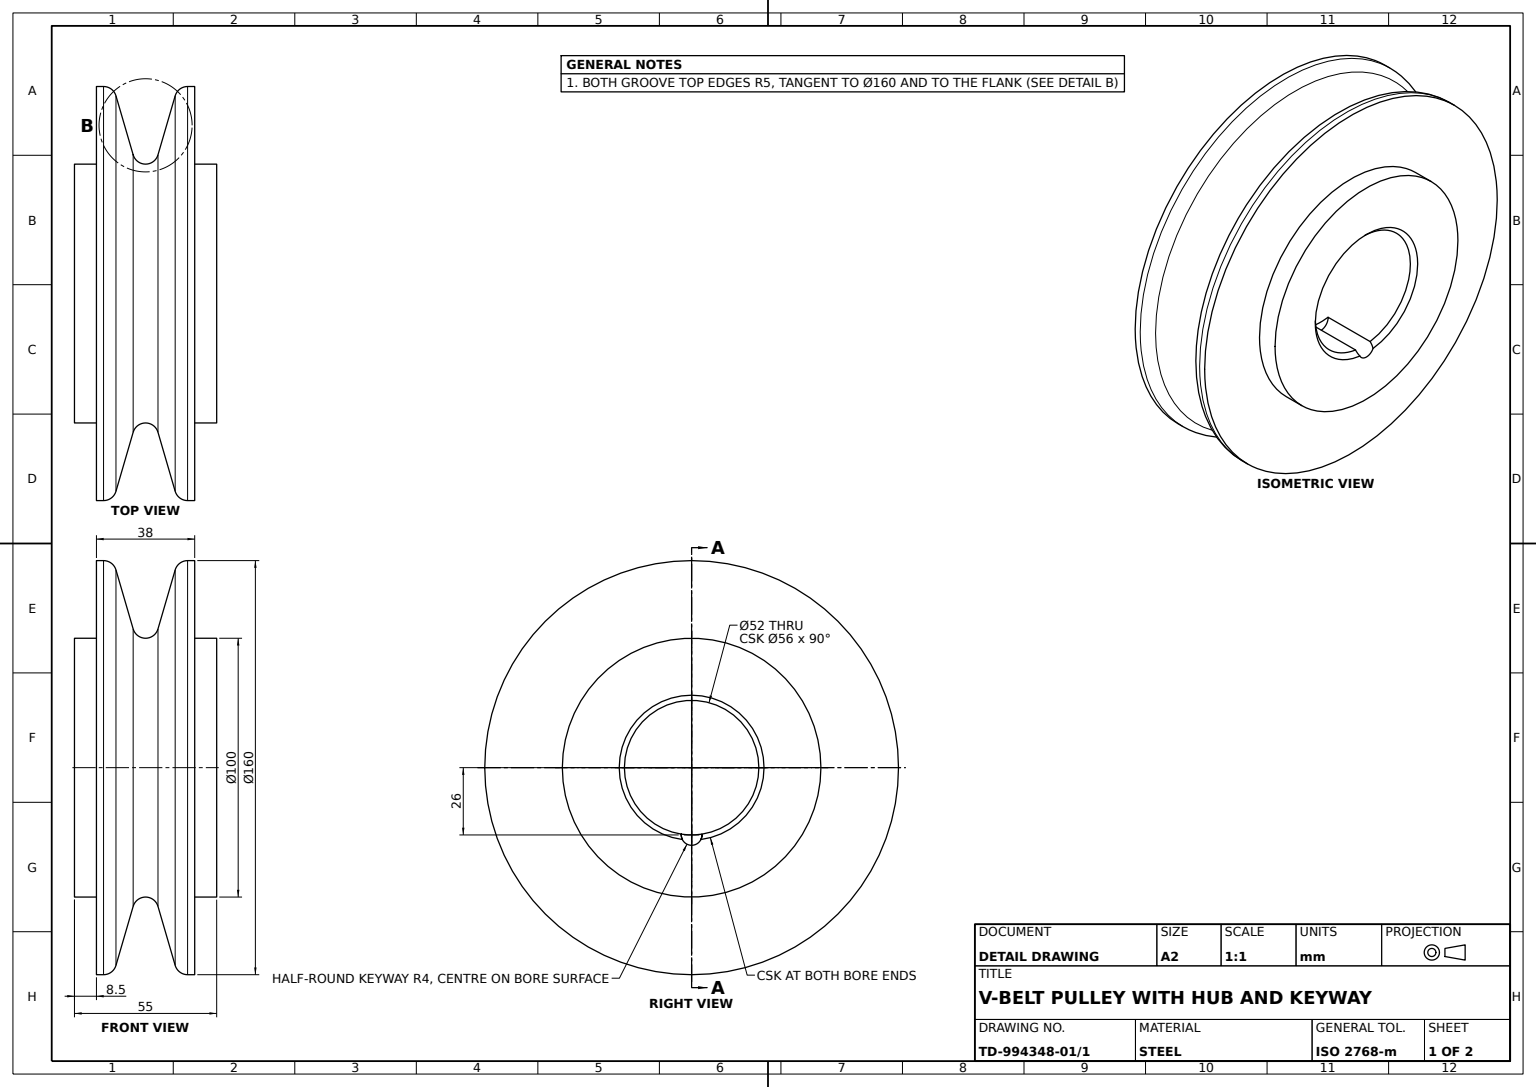
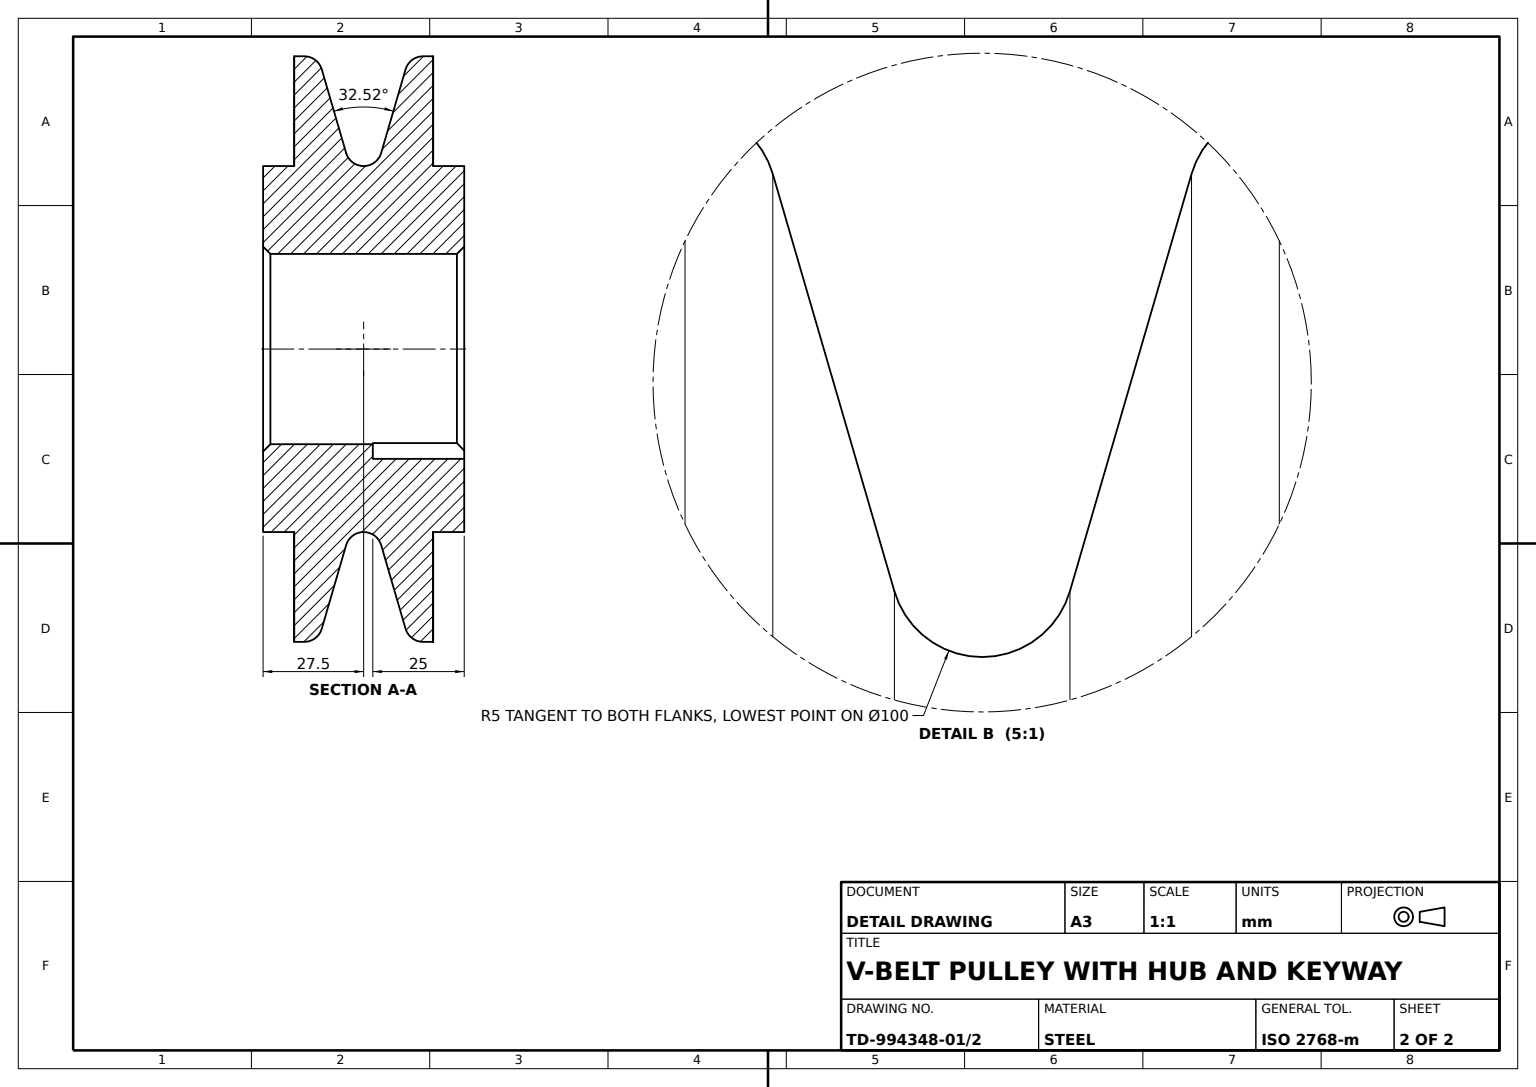
from build123d import *

# Parameters (mm, degrees)
EDGE_CHAMFER_2MM_SIZE = 2
KEYWAY_SKETCH_R       = 4
KEYWAY_CUT_8MM_DEPTH  = 25


with BuildPart() as part:
    # Pulley Profile Sketch → Pulley Body (revolve)
    with BuildSketch(Plane.XY, mode=Mode.PRIVATE) as pulley_body_sk:
        with BuildLine():
            Line((-27.5, 26), (27.5, 26))
            Line((27.5, 26), (27.5, 50))
            Line((27.5, 50), (19, 50))
            Line((19, 50), (19, 80))
            Line((19, 80), (16.25, 80))
            ThreePointArc((16.25, 80), (13.25, 79), (11.45, 76.4))
            Line((11.45, 76.4), (4.8, 53.6))
            ThreePointArc((4.8, 53.6), (0, 50), (-4.8, 53.6))
            Line((-4.8, 53.6), (-11.45, 76.4))
            ThreePointArc((-11.45, 76.4), (-13.25, 79), (-16.25, 80))
            Line((-16.25, 80), (-19, 80))
            Line((-19, 80), (-19, 50))
            Line((-19, 50), (-27.5, 50))
            Line((-27.5, 50), (-27.5, 26))
        make_face()
    revolve(pulley_body_sk.sketch.rotate(Axis((0, 0, 0), (1, 0, 0)), 90), axis=Axis((0, 0, 0), (1, 0, 0)))

    # Edge Chamfer 2mm
    edge_chamfer_2mm_edges = [part.edges().sort_by_distance(p)[0] for p in [
        (27.5, 0, -26),
        (-27.5, 0, -26),
    ]]
    chamfer(edge_chamfer_2mm_edges, length=EDGE_CHAMFER_2MM_SIZE)

    # Keyway Sketch → Keyway Cut 8mm (cut)
    with BuildSketch(Plane(origin=(27.5, 0, 0), x_dir=(0, 0, -1), z_dir=(1, 0, 0))):
        with Locations((0, -26)):
            Circle(KEYWAY_SKETCH_R)
    extrude(amount=-KEYWAY_CUT_8MM_DEPTH, mode=Mode.SUBTRACT)


solid = part.part
